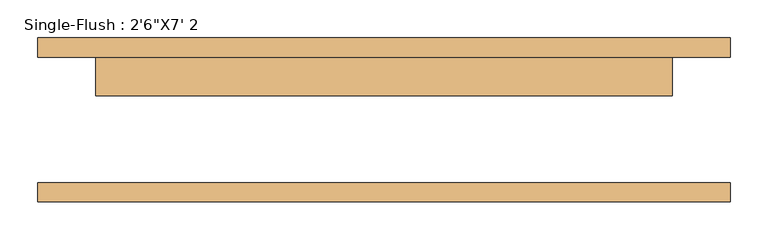
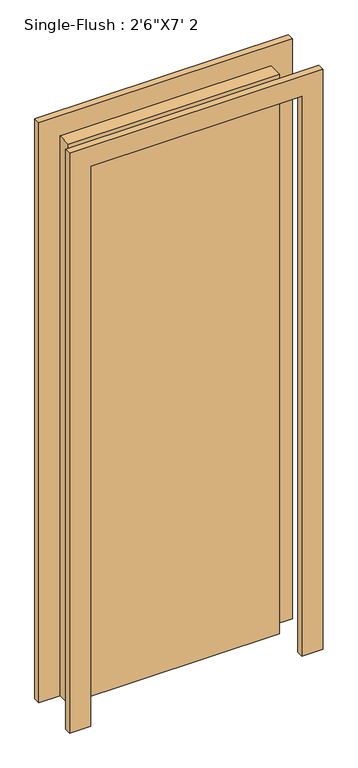
"""IFC4 building model written with IfcOpenShell, lengths in millimetres: door geometry."""

from ifc_helpers import new_model, si_unit, frame, origin, origin_with_axes, place, context, project, spatial, polyline, outline, extrude, source, transform, mapped, element, save


def door_9181f8a1(model_context):
    return source(origin(), model_context, "Body", "SweptSolid", [
        extrude(outline(polyline([(2209.8, -457.2), (0.0, -457.2), (0.0, -381.0), (2133.6, -381.0), (2133.6, 381.0), (0.0, 381.0), (0.0, 457.2), (2209.8, 457.2), (2209.8, -457.2)])), frame((0.0, 82.9, 0.0), z_axis=(0.0, 1.0, 0.0), x_axis=(0.0, 0.0, 1.0)), (0.0, 0.0, 1.0), 25.4),
        extrude(outline(polyline([(2209.8, 457.2), (2209.8, -457.2), (0.0, -457.2), (0.0, -381.0), (2133.6, -381.0), (2133.6, 381.0), (0.0, 381.0), (0.0, 457.2), (2209.8, 457.2)])), frame((0.0, -108.3, 0.0), z_axis=(0.0, 1.0, 0.0), x_axis=(0.0, 0.0, 1.0)), (0.0, 0.0, 1.0), 25.4),
        extrude(outline(polyline([(381.0, 32.1), (-381.0, 32.1), (-381.0, 82.9), (381.0, 82.9), (381.0, 32.1)])), origin_with_axes(), (0.0, 0.0, 1.0), 2133.6),
    ])


if __name__ == "__main__":
    model = new_model("IFC4")
    model_context = context("Model", 3, world=origin())
    ifc_project = project(units=[si_unit("LENGTHUNIT", "METRE", prefix="MILLI")], contexts=[model_context])
    site = spatial("IfcSite", under=ifc_project)
    building = spatial("IfcBuilding", under=site)
    placement = place(None, origin())
    door_shape = door_9181f8a1(model_context)
    element("IfcDoor", 1, ObjectType="Single-Flush : 2'6\"X7' 2", at=placement, inside=building, context=model_context, shape_type="MappedRepresentation", body=[
        mapped(door_shape, transform((0.0, 0.0, 0.0), x_axis=(1.0, 0.0, 0.0), y_axis=(0.0, 1.0, 0.0), z_axis=(0.0, 0.0, 1.0))),
    ])
    save(model, "model.ifc")

# Revit data of these elements
# Type "Single-Flush : 2'6\"X7' 2"
#   Type Mark = "9"
#   Assembly Code = "C1020"
#   Thickness = 0' - 2"
#   Height = 7' - 0"
#   Trim Projection Ext = 0' - 1"
#   Trim Projection Int = 0' - 1"
#   Trim Width = 0' - 3"
#   Width = 2' - 6"
#   Door Material = Door - Panel
#   Frame Material = Door - Frame
#   Function = (empty or 0)
#   Wall Closure = (empty or 0)
# Element 1 (IfcDoor, "Single-Flush : 2'6\"X7' 2")
#   Materials on its faces: "Door - Frame", "Door - Panel"
# Materials
#   "Door - Panel": class "Wood", colour RGB 114 82 51, transparency 0
#   "Door - Frame": colour RGB 153 76 43, transparency 0
